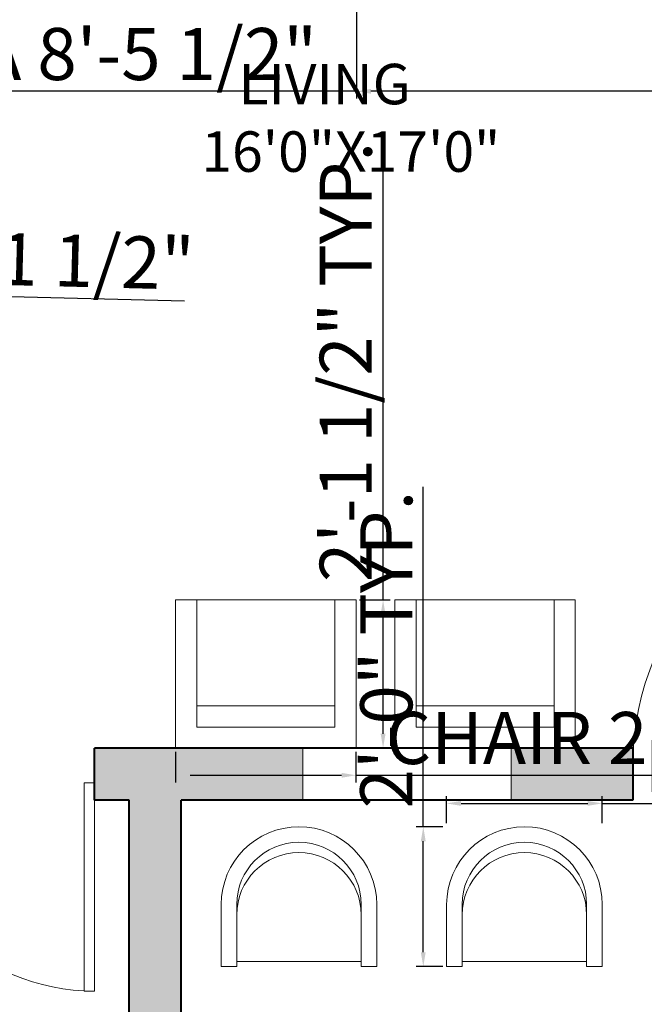
# Model space of a CAD drawing. Units: inches. Extents: x 2337 to 3570, y 1258 to 1938.
# Tile 6 of 30: x 2704 to 2812, y 1507 to 1677. Entities that reach past the tile are written whole.
import ezdxf

# ---------------------------------------------------------------- set-up
doc = ezdxf.new("R2010")
doc.units = ezdxf.units.IN
for name, color, linetype, lineweight in [('A-ANNO-DIMS', 2, 'Continuous', 18), ('A-AREA-IDEN', 7, 'Continuous', 18), ('A-DOOR', 4, 'Continuous', 20), ('A-GLAZ', 4, 'Continuous', 18), ('A-WALL', 7, 'Continuous', 40), ('furn', 8, 'Continuous', 18)]:
    doc.layers.add(name, color=color, linetype=linetype, lineweight=lineweight)
doc.layers.add('A-WALL-PATT', color=18, linetype='Continuous', lineweight=13, true_color=0x000000)
doc.styles.get("Standard").update_dxf_attribs({"font": 'arial.ttf'})
doc.dimstyles.new('ISO-25', dxfattribs={"dimtxt": 9, "dimasz": 2.5, "dimexe": 1.25, "dimexo": 0.625, "dimtad": 1, "dimdec": 1, "dimlunit": 3, "dimtxsty": 'Standard', "dimcen": 2.5, "dimadec": 0, "dimazin": 0, "dimtfac": 1, "dimtdec": 1, "dimtmove": 0, "dimatfit": 3, "dimfxl": 1, "dimarcsym": 0})

# ---------------------------------------------------------------- blocks, each defined once
blk = doc.blocks.new('*U2')
for p, q in [((0, 0), (0, -6)), ((36, 0), (36, -6))]:
    blk.add_line(p, q)
blk.add_lwpolyline([(0, 0), (0, 36), (1.75, 36), (1.75, 0)], close=True)
blk.add_arc((0, 0), 36, 0, 90)
blk = doc.blocks.new('A$C5A6E6C9E')
at = {"layer": 'furn'}
for p, q in [((0.0001, 0), (0, 0.3658)), ((0.0914, 0.3658), (0.0916, 0)), ((0.823, 0.3661), (0.8231, 0.0003)), ((0.9145, 0.0004), (0.9144, 0.3661)), ((0.0916, 0), (0.0001, 0)), ((0.8231, 0.0308), (0.0916, 0.0305)), ((0.8231, 0.0003), (0.9145, 0.0004))]:
    blk.add_line(p, q, dxfattribs=at)
for centre, radius in [((0.4572, 0.3659), 0.4572), ((0.4572, 0.3659), 0.3658), ((0.4572, 0.305), 0.3658)]:
    blk.add_arc(centre, radius, 0.02324, 180.02324, dxfattribs=at)
blk = doc.blocks.new('sofa-10')
at = {"color": 0, "linetype": 'ByBlock'}
for p, q in [((0, 0.7), (0, 0)), ((0.85, 0.7), (0, 0.7)), ((0.1, 0.7), (0.1, 0.1)), ((0.75, 0.1), (0.75, 0.7)), ((0.85, 0), (0.85, 0.7)), ((0.1, 0.2), (0.75, 0.2)), ((0.1, 0.1), (0.75, 0.1)), ((0, 0), (0.85, 0))]:
    blk.add_line(p, q, dxfattribs=at)
blk = doc.blocks.new('DOOR-SWING-48IN')
for p, q in [((0, 6), (0, 0)), ((48, 6), (48, 0))]:
    blk.add_line(p, q)
blk.add_lwpolyline([(48, 6), (48, 54), (46.25, 54), (46.25, 6)], close=True)
blk.add_arc((48, 6), 48, 90, 180)
blk = doc.blocks.new('*D50')
at = {"layer": 'A-ANNO-DIMS', "color": 0, "lineweight": -2, "transparency": 16777216}
for p, q in [((2777.67, 1538.17), (2777.67, 1542.83)), ((2804.55, 1538.17), (2804.55, 1542.83)), ((2780.17, 1541.58), (2802.05, 1541.58)), ((2804.55, 1541.58), (2954.22, 1541.58))]:
    blk.add_line(p, q, dxfattribs=at)
at = {"layer": 'A-ANNO-DIMS', "color": 0, "transparency": 16777216}
for points in [[(2780.17, 1542), (2780.17, 1541.16), (2777.67, 1541.58)], [(2802.05, 1542), (2802.05, 1541.16), (2804.55, 1541.58)]]:
    blk.add_solid(points, dxfattribs=at)
at = {"layer": 'Defpoints', "color": 0, "transparency": 16777216}
for p in [(2804.55, 1541.58), (2777.67, 1537.55), (2804.55, 1537.55)]:
    blk.add_point(p, dxfattribs=at)
at = {"layer": 'A-ANNO-DIMS', "color": 0, "transparency": 16777216, "insert": (2880.63, 1546.87), "char_height": 9, "attachment_point": 5}
blk.add_mtext('PORCH CHAIR 2\'-3" TYP.', dxfattribs=at)
blk = doc.blocks.new('*D51')
at = {"layer": 'A-ANNO-DIMS', "color": 0, "lineweight": -2, "transparency": 16777216}
for p, q in [((2773.64, 1537.55), (2773.64, 1596.31)), ((2777.05, 1537.55), (2772.39, 1537.55)), ((2773.64, 1515.86), (2773.64, 1535.05)), ((2777.05, 1513.36), (2772.39, 1513.36))]:
    blk.add_line(p, q, dxfattribs=at)
at = {"layer": 'A-ANNO-DIMS', "color": 0, "transparency": 16777216}
for points in [[(2773.22, 1535.05), (2774.06, 1535.05), (2773.64, 1537.55)], [(2773.22, 1515.86), (2774.06, 1515.86), (2773.64, 1513.36)]]:
    blk.add_solid(points, dxfattribs=at)
at = {"layer": 'Defpoints', "color": 0, "transparency": 16777216}
for p in [(2773.64, 1537.55), (2777.67, 1537.55), (2777.67, 1513.36)]:
    blk.add_point(p, dxfattribs=at)
at = {"layer": 'A-ANNO-DIMS', "color": 0, "transparency": 16777216, "insert": (2768.42, 1568.18), "char_height": 9, "attachment_point": 5, "rotation": 90}
blk.add_mtext('2\'-0" TYP.', dxfattribs=at)
blk = doc.blocks.new('*D52')
at = {"layer": 'A-ANNO-DIMS', "color": 0, "lineweight": -2, "transparency": 16777216}
for p, q in [((2730.86, 1550.49), (2730.86, 1545.19)), ((2762.02, 1550.49), (2762.02, 1545.19)), ((2733.36, 1546.44), (2759.52, 1546.44)), ((2762.02, 1546.44), (2863.14, 1546.44))]:
    blk.add_line(p, q, dxfattribs=at)
at = {"layer": 'A-ANNO-DIMS', "color": 0, "transparency": 16777216}
for points in [[(2733.36, 1546.86), (2733.36, 1546.02), (2730.86, 1546.44)], [(2759.52, 1546.86), (2759.52, 1546.02), (2762.02, 1546.44)]]:
    blk.add_solid(points, dxfattribs=at)
at = {"layer": 'Defpoints', "color": 0, "transparency": 16777216}
for p in [(2730.86, 1551.12), (2762.02, 1551.12), (2762.02, 1546.44)]:
    blk.add_point(p, dxfattribs=at)
at = {"layer": 'A-ANNO-DIMS', "color": 0, "transparency": 16777216, "insert": (2813.83, 1551.72), "char_height": 9, "attachment_point": 5}
blk.add_mtext('CHAIR 2\'-7" TYP.', dxfattribs=at)
blk = doc.blocks.new('*D53')
at = {"layer": 'A-ANNO-DIMS', "color": 0, "lineweight": -2, "transparency": 16777216}
for p, q in [((2766.7, 1576.78), (2766.7, 1656.52)), ((2762.65, 1576.78), (2767.95, 1576.78)), ((2766.7, 1553.62), (2766.7, 1574.28)), ((2762.65, 1551.12), (2767.95, 1551.12))]:
    blk.add_line(p, q, dxfattribs=at)
at = {"layer": 'A-ANNO-DIMS', "color": 0, "transparency": 16777216}
for points in [[(2766.28, 1574.28), (2767.12, 1574.28), (2766.7, 1576.78)], [(2766.28, 1553.62), (2767.12, 1553.62), (2766.7, 1551.12)]]:
    blk.add_solid(points, dxfattribs=at)
at = {"layer": 'Defpoints', "color": 0, "transparency": 16777216}
for p in [(2762.02, 1576.78), (2766.7, 1576.78), (2762.02, 1551.12)]:
    blk.add_point(p, dxfattribs=at)
at = {"layer": 'A-ANNO-DIMS', "color": 0, "transparency": 16777216, "insert": (2761.42, 1617.9), "char_height": 9, "attachment_point": 5, "rotation": 90}
blk.add_mtext('2\'-1 1/2" TYP.', dxfattribs=at)
blk = doc.blocks.new('*D55')
at = {"layer": 'A-ANNO-DIMS', "color": 0, "lineweight": -2, "transparency": 16777216}
for p, q in [((2671.13, 1636.16), (2670.94, 1628.78)), ((2684.79, 1635.82), (2684.6, 1628.43)), ((2673.47, 1629.97), (2682.14, 1629.74)), ((2684.64, 1629.68), (2732.42, 1628.47))]:
    blk.add_line(p, q, dxfattribs=at)
at = {"layer": 'A-ANNO-DIMS', "color": 0, "transparency": 16777216}
for points in [[(2673.48, 1630.38), (2673.46, 1629.55), (2670.97, 1630.03)], [(2682.15, 1630.16), (2682.13, 1629.33), (2684.64, 1629.68)]]:
    blk.add_solid(points, dxfattribs=at)
at = {"layer": 'Defpoints', "color": 0, "transparency": 16777216}
for p in [(2671.14, 1636.79), (2684.81, 1636.44), (2684.64, 1629.68)]:
    blk.add_point(p, dxfattribs=at)
at = {"layer": 'A-ANNO-DIMS', "color": 0, "transparency": 16777216, "insert": (2709.91, 1634.32), "char_height": 9, "attachment_point": 5, "rotation": 358.5431}
blk.add_mtext('1\'-1 1/2"', dxfattribs=at)
blk = doc.blocks.new('*D65')
at = {"layer": 'A-ANNO-DIMS', "color": 0, "lineweight": -2, "transparency": 16777216}
for p, q in [((2756.86, 1473.54), (2756.86, 1496)), ((2759.36, 1494.75), (2814.09, 1494.75)), ((2816.59, 1473.54), (2816.59, 1496)), ((2816.59, 1494.75), (2903.52, 1494.75))]:
    blk.add_line(p, q, dxfattribs=at)
at = {"layer": 'A-ANNO-DIMS', "color": 0, "transparency": 16777216}
for points in [[(2759.36, 1495.17), (2759.36, 1494.34), (2756.86, 1494.75)], [(2814.09, 1495.17), (2814.09, 1494.34), (2816.59, 1494.75)]]:
    blk.add_solid(points, dxfattribs=at)
at = {"layer": 'Defpoints', "color": 0, "transparency": 16777216}
for p in [(2816.59, 1494.75), (2756.86, 1472.91), (2816.59, 1472.91)]:
    blk.add_point(p, dxfattribs=at)
at = {"layer": 'A-ANNO-DIMS', "color": 0, "transparency": 16777216, "insert": (2861.3, 1500.03), "char_height": 9, "attachment_point": 5}
blk.add_mtext('4\'-11 1/2" TYP.', dxfattribs=at)
blk = doc.blocks.new('*D86')
at = {"layer": 'A-ANNO-DIMS', "color": 0, "lineweight": -2, "transparency": 16777216}
for p, q in [((2762.09, 1679.33), (2762.09, 1663.44)), ((2863.84, 1679.33), (2863.84, 1663.44)), ((2762.09, 1664.69), (2617.85, 1664.69)), ((2861.34, 1664.69), (2764.59, 1664.69))]:
    blk.add_line(p, q, dxfattribs=at)
at = {"layer": 'A-ANNO-DIMS', "color": 0, "transparency": 16777216}
for points in [[(2764.59, 1665.11), (2764.59, 1664.28), (2762.09, 1664.69)], [(2861.34, 1665.11), (2861.34, 1664.28), (2863.84, 1664.69)]]:
    blk.add_solid(points, dxfattribs=at)
at = {"layer": 'Defpoints', "color": 0, "transparency": 16777216}
for p in [(2762.09, 1679.95), (2863.84, 1679.95), (2762.09, 1664.69)]:
    blk.add_point(p, dxfattribs=at)
at = {"layer": 'A-ANNO-DIMS', "color": 0, "transparency": 16777216, "insert": (2688.72, 1669.97), "char_height": 9, "attachment_point": 5}
blk.add_mtext('CORNER SOFA 8\'-5 1/2"', dxfattribs=at)

msp = doc.modelspace()

# ---------------------------------------------------------------- hatches: boundary and pattern name
at = {"layer": 'A-WALL-PATT'}
h = msp.add_hatch(color=256, dxfattribs=at)
h.dxf.hatch_style = 1
h.paths.add_polyline_path([(2671.84, 1857.12), (2455.84, 1857.12), (2455.84, 1824.12), (2464.84, 1824.12), (2464.84, 1848.12), (2671.84, 1848.12)])
h.paths.add_polyline_path([(2566.84, 1764.12), (2464.84, 1764.12), (2464.84, 1788.12), (2455.84, 1788.12), (2455.84, 1743.12), (2464.84, 1743.12), (2464.84, 1755.12), (2566.84, 1755.12)])
h.paths.add_polyline_path([(2683.84, 1761.12), (2683.84, 1764.12), (2602.84, 1764.12), (2602.84, 1755.12), (2608.84, 1755.12), (2608.84, 1701.12), (2662.84, 1701.12), (2662.84, 1605.12), (2671.84, 1605.12), (2671.84, 1713.12), (2662.84, 1713.12), (2662.84, 1707.12), (2614.84, 1707.12), (2614.84, 1755.12), (2662.84, 1755.12), (2662.84, 1749.12), (2671.84, 1749.12), (2671.84, 1755.12), (2683.84, 1755.12)])
h.paths.add_polyline_path([(2464.84, 1707.12), (2455.84, 1707.12), (2455.84, 1617.12), (2464.84, 1617.12), (2464.84, 1635.12), (2506.84, 1635.12), (2506.84, 1641.12), (2464.84, 1641.12)])
h.paths.add_polyline_path([(2542.84, 1551.12), (2464.84, 1551.12), (2464.84, 1569.12), (2455.84, 1569.12), (2455.84, 1518.12), (2464.84, 1518.12), (2464.84, 1542.12), (2542.84, 1542.12)])
h.paths.add_polyline_path([(2464.84, 1482.12), (2455.84, 1482.12), (2455.84, 1410.12), (2464.84, 1410.12)])
h.paths.add_polyline_path([(2626.84, 1350.12), (2590.84, 1350.12), (2590.84, 1380.12), (2584.84, 1380.12), (2584.84, 1350.12), (2464.84, 1350.12), (2464.84, 1374.12), (2455.84, 1374.12), (2455.84, 1341.12), (2626.84, 1341.12)])
h.paths.add_polyline_path([(2662.84, 1416.12), (2686.84, 1416.12), (2686.84, 1422.12), (2590.84, 1422.12), (2590.84, 1542.12), (2680.84, 1542.12), (2680.84, 1551.12), (2671.84, 1551.12), (2671.84, 1557.12), (2662.84, 1557.12), (2662.84, 1551.12), (2578.84, 1551.12), (2578.84, 1542.12), (2584.84, 1542.12), (2584.84, 1410.12), (2590.84, 1410.12), (2590.84, 1416.12), (2656.84, 1416.12), (2656.84, 1350.12), (2650.84, 1350.12), (2650.84, 1341.12), (2731.84, 1341.12), (2731.84, 1362.12), (2722.84, 1362.12), (2722.84, 1350.12), (2662.84, 1350.12)])
h.paths.add_polyline_path([(2731.84, 1434.12), (2722.84, 1434.12), (2722.84, 1422.12), (2716.84, 1422.12), (2716.84, 1416.12), (2722.84, 1416.12), (2722.84, 1386.12), (2731.84, 1386.12)], flags=17)
h.paths.add_polyline_path([(2731.84, 1542.12), (2752.84, 1542.12), (2752.84, 1551.12), (2716.84, 1551.12), (2716.84, 1545.12), (2716.84, 1542.12), (2722.84, 1542.12), (2722.84, 1482.12), (2731.84, 1482.12)])
h.paths.add_polyline_path([(2809.84, 1551.12), (2788.84, 1551.12), (2788.84, 1542.12), (2809.84, 1542.12), (2809.84, 1548.12)])
h.paths.add_polyline_path([(2872.84, 1647.12), (2863.84, 1647.12), (2863.84, 1551.12), (2857.84, 1551.12), (2857.84, 1548.12), (2857.84, 1542.12), (2872.84, 1542.12)])
h.paths.add_polyline_path([(2872.84, 1764.12), (2827.84, 1764.12), (2827.84, 1755.12), (2863.84, 1755.12), (2863.84, 1719.12), (2872.84, 1719.12)])
h.paths.add_polyline_path([(2755.84, 1764.12), (2719.84, 1764.12), (2719.84, 1755.12), (2755.84, 1755.12)])

# ---------------------------------------------------------------- linework, layer by layer
at = {"layer": 'A-GLAZ'}
for p, q in [((2752.84, 1542.12), (2752.84, 1551.12)), ((2788.84, 1542.12), (2788.84, 1551.12))]:
    msp.add_line(p, q, dxfattribs=at)
at = {"layer": 'A-WALL'}
for p, q in [((2809.84, 1551.12), (2716.84, 1551.12)), ((2716.84, 1542.12), (2716.84, 1551.12)), ((2809.84, 1551.12), (2809.84, 1542.12)), ((2722.84, 1542.12), (2716.84, 1542.12)), ((2722.84, 1422.12), (2722.84, 1542.12)), ((2809.84, 1542.12), (2731.84, 1542.12)), ((2731.84, 1341.12), (2731.84, 1542.12))]:
    msp.add_line(p, q, dxfattribs=at)

# ---------------------------------------------------------------- block references
at = {"layer": 'A-DOOR'}
msp.add_blockref('DOOR-SWING-48IN', (2809.84, 1542.12), dxfattribs=at)
at = {"layer": 'A-DOOR', "rotation": 180}
msp.add_blockref('*U2', (2716.84, 1545.12), dxfattribs=at)
at = {"layer": 'furn'}
for name, p, xscale, yscale, zscale in [('sofa-10', (2730.86, 1551.12), 36.66436083614781, 36.66436083614781, 36.66436083614781), ('sofa-10', (2768.74, 1551.12), 36.66436083614781, 36.66436083614781, 36.66436083614781), ('A$C5A6E6C9E', (2738.74, 1513.36), 29.38291643341122, 29.38291643341122, 29.38291643341122), ('A$C5A6E6C9E', (2777.68, 1513.36), 29.38291643341122, 29.38291643341122, 29.38291643341122)]:
    msp.add_blockref(name, p, dxfattribs=dict(at, xscale=xscale, yscale=yscale, zscale=zscale))

# ---------------------------------------------------------------- texts
at = {"layer": 'A-AREA-IDEN', "insert": (2735.31, 1669.44), "char_height": 7, "attachment_point": 1}
msp.add_mtext_dynamic_manual_height_columns('   LIVING\\P16\'0"X17\'0"', width=66.911, gutter_width=12.5, heights=[0], dxfattribs=at)

# ---------------------------------------------------------------- dimensions: what is measured, and where the dimension line sits
at = {"layer": 'A-ANNO-DIMS'}
for base, p1, p2, angle, text, picture, middle in [((2762.0922, 1664.6925), (2863.8358, 1679.9541), (2762.0922, 1679.9541), 180, 'CORNER SOFA <>', '*D86', (2688.7199, 1669.9741)), ((2766.7, 1576.78), (2762.02, 1551.12), (2762.02, 1576.78), 90, '<> TYP.', '*D53', (2761.42, 1617.9)), ((2773.64, 1537.55), (2777.67, 1513.36), (2777.67, 1537.55), 90, '<> TYP.', '*D51', (2768.42, 1568.18))]:
    dim = msp.add_linear_dim(base=base, p1=p1, p2=p2, angle=angle, text=text, dimstyle='ISO-25', override={"dimdec": 1, "dimlfac": 1, "dimrnd": 0, "dimzin": 1, "dimdsep": 46, "dimlunit": 4, "dimfrac": 2}, dxfattribs=at)
    dim.commit()
    dim.dimension.update_dxf_attribs({"geometry": picture, "text_midpoint": middle})
dim = msp.add_linear_dim(base=(2684.64, 1629.68), p1=(2671.14, 1636.79), p2=(2684.81, 1636.44), angle=358.5431, dimstyle='ISO-25', override={"dimdec": 1, "dimlfac": 1, "dimrnd": 0, "dimzin": 1, "dimdsep": 46, "dimlunit": 4, "dimfrac": 2}, dxfattribs=at)
dim.commit()
dim.dimension.update_dxf_attribs({"geometry": '*D55', "text_midpoint": (2709.91, 1634.32)})
for base, p1, p2, text, picture, middle in [((2804.55, 1541.58), (2777.67, 1537.55), (2804.55, 1537.55), 'PORCH CHAIR <> TYP.', '*D50', (2880.63, 1546.87)), ((2762.02, 1546.44), (2730.86, 1551.12), (2762.02, 1551.12), 'CHAIR <> TYP.', '*D52', (2813.83, 1551.72)), ((2816.59, 1494.75), (2756.86, 1472.91), (2816.59, 1472.91), '<> TYP.', '*D65', (2861.3, 1500.03))]:
    dim = msp.add_linear_dim(base=base, p1=p1, p2=p2, text=text, dimstyle='ISO-25', override={"dimdec": 1, "dimlfac": 1, "dimrnd": 0, "dimzin": 1, "dimdsep": 46, "dimlunit": 4, "dimfrac": 2}, dxfattribs=at)
    dim.commit()
    dim.dimension.update_dxf_attribs({"geometry": picture, "text_midpoint": middle})

doc.saveas('drawing.dxf')
